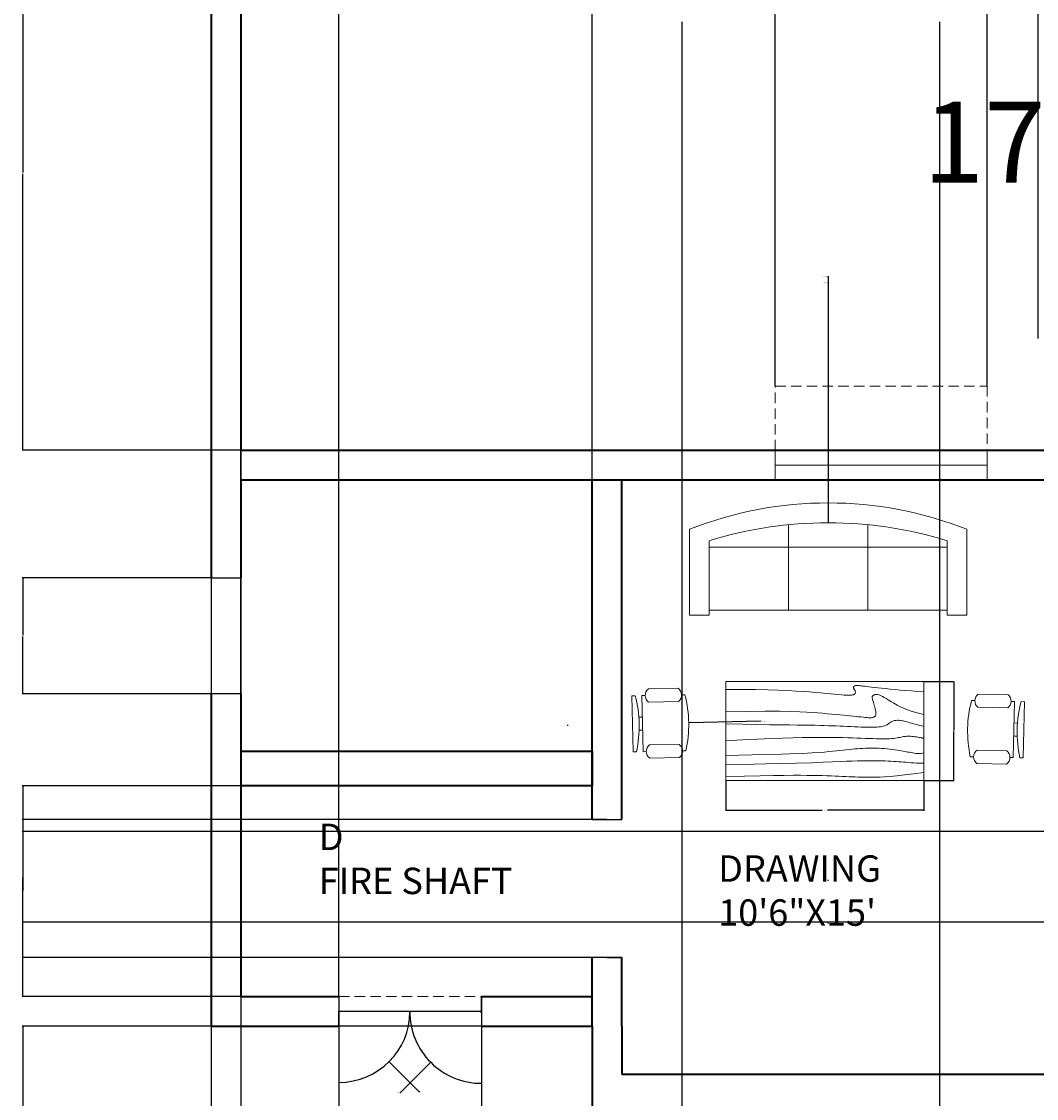
# Model space of a CAD drawing. Units: inches. Extents: x 276 to 912, y -567 to 621.
# Tile 2 of 7: x 276 to 583, y -261 to 65. Entities that reach past the tile are written whole.
import ezdxf

# ---------------------------------------------------------------- set-up
doc = ezdxf.new("R2010")
doc.units = ezdxf.units.IN
doc.linetypes.add('HIDDEN2', pattern=[4.7625, 3.175, -1.5875])
for name, color, linetype, lineweight in [('A-ANNO-DIMS', 2, 'Continuous', 18), ('A-ANNO-TEXT', 7, 'Continuous', 35), ('A-AREA-IDEN', 7, 'Continuous', 18), ('A-DOOR', 3, 'Continuous', 25), ('A-DOOR-HIDN', 3, 'HIDDEN2', 18), ('A-FLOR-OVHD', 8, 'HIDDEN2', 13), ('A-FURN', 8, 'Continuous', 18), ('A-GLAZ', 4, 'Continuous', 18), ('A-WALL', 7, 'Continuous', 35)]:
    doc.layers.add(name, color=color, linetype=linetype, lineweight=lineweight)
doc.dimstyles.get("Standard").update_dxf_attribs({"dimtxt": 0.18, "dimasz": 0.18, "dimexe": 0.18, "dimexo": 0.0625, "dimgap": 0.09, "dimtad": 0, "dimtih": 1, "dimtoh": 1, "dimdec": 4, "dimzin": 0, "dimdsep": 46, "dimtxsty": 'Standard', "dimcen": 0.09, "dimadec": 0, "dimazin": 0, "dimtfac": 1, "dimtdec": 4, "dimtofl": 0, "dimtmove": 0, "dimatfit": 3, "dimfxl": 1, "dimtolj": 1, "dimtzin": 0, "dimarcsym": 0})

# ---------------------------------------------------------------- blocks, each defined once
blk = doc.blocks.new('Table - Rectangular Woodgrain 60 x 30 in.')
for p, q in [((0, 0), (0, -30)), ((60, 0), (0, 0)), ((60, -30), (60, 0)), ((0, -30), (60, -30))]:
    blk.add_line(p, q)
for points in [[(0, -2.4), (4.8155, -2.418), (9.0302, -2.4688), (12.709, -2.5477), (15.9167, -2.65), (18.7181, -2.7711), (21.1781, -2.9063), (23.3616, -3.0508), (25.3333, -3.2), (27.1477, -3.3495), (28.8172, -3.4958), (30.3437, -3.636), (31.7291, -3.7667), (32.9756, -3.8849), (34.0849, -3.9875), (35.059, -4.0714), (35.9, -4.1334), (36.6114, -4.1711), (37.2041, -4.1854), (37.6906, -4.1779), (38.0833, -4.15), (38.3948, -4.1034), (38.6375, -4.0396), (38.8239, -3.9602), (38.9666, -3.8667), (39.0764, -3.7608), (39.1573, -3.6448), (39.2116, -3.521), (39.2416, -3.3917), (39.2498, -3.2593), (39.2385, -3.1261), (39.21, -2.9944), (39.1666, -2.8667), (39.111, -2.7447), (39.0468, -2.6281), (38.978, -2.5163), (38.9083, -2.4083), (38.8418, -2.3035), (38.7823, -2.201), (38.7337, -2.1001), (38.7, -2), (38.6844, -1.9003), (38.6875, -1.8021), (38.7094, -1.707), (38.75, -1.6167), (38.8094, -1.5326), (38.8875, -1.4563), (38.9844, -1.3893), (39.1, -1.3333), (39.2351, -1.2896), (39.3937, -1.2583), (39.5804, -1.2396), (39.8, -1.2333), (40.057, -1.2396), (40.3562, -1.2583), (40.7023, -1.2896), (41.1, -1.3333), (41.5547, -1.3895), (42.0755, -1.4573), (42.6721, -1.5361), (43.3542, -1.625), (44.1316, -1.7233), (45.014, -1.8302), (46.0114, -1.9449), (47.1333, -2.0667), (48.3862, -2.1947), (49.7625, -2.3281), (51.2513, -2.4663), (52.8416, -2.6083), (54.5226, -2.7535), (56.2833, -2.9011), (58.1127, -3.0501), (60, -3.2)], [(0, -9.2), (6.5759, -9.0858), (11.9385, -9.0365), (16.2527, -9.0418), (19.6833, -9.0917), (22.3952, -9.1759), (24.5531, -9.2844), (26.322, -9.4069), (27.8666, -9.5333), (29.3241, -9.6553), (30.7203, -9.7719), (32.0532, -9.8837), (33.3208, -9.9917), (34.5213, -10.0965), (35.6526, -10.199), (36.7128, -10.2999), (37.7, -10.4), (38.6129, -10.4996), (39.4531, -10.5969), (40.223, -10.6895), (40.925, -10.775), (41.5613, -10.8512), (42.1344, -10.9156), (42.6465, -10.966), (43.1, -11), (43.4976, -11.0158), (43.8437, -11.0136), (44.143, -10.9942), (44.4, -10.9583), (44.6195, -10.9069), (44.8062, -10.8406), (44.9648, -10.7603), (45.1, -10.6667), (45.2155, -10.5598), (45.3114, -10.4365), (45.3871, -10.2929), (45.4416, -10.125), (45.4743, -9.929), (45.4844, -9.7011), (45.4709, -9.4371), (45.4333, -9.1333), (45.3716, -8.7883), (45.2896, -8.4104), (45.1919, -8.0107), (45.0833, -7.6), (44.9685, -7.1893), (44.8521, -6.7896), (44.7388, -6.4117), (44.6333, -6.0667), (44.54, -5.7628), (44.4614, -5.4979), (44.4001, -5.2675), (44.3583, -5.0667), (44.3384, -4.8909), (44.3427, -4.7354), (44.3736, -4.5956), (44.4333, -4.4667), (44.5236, -4.3453), (44.6427, -4.2333), (44.7884, -4.1339), (44.9583, -4.05), (45.1501, -3.9849), (45.3614, -3.9417), (45.59, -3.9234), (45.8333, -3.9333), (46.0915, -3.9749), (46.3734, -4.0531), (46.6906, -4.1736), (47.0542, -4.3417), (47.4756, -4.5629), (47.9661, -4.8427), (48.5372, -5.1866), (49.2, -5.6), (49.9676, -6.0844), (50.8594, -6.625), (51.8965, -7.2031), (53.1, -7.8), (54.491, -8.3969), (56.0906, -8.975), (57.9199, -9.5156), (60, -10)], [(0, -12.8), (5.1847, -12.9322), (9.6213, -13.0323), (13.3963, -13.1059), (16.5958, -13.1583), (19.3063, -13.1952), (21.614, -13.2219), (23.6054, -13.2439), (25.3666, -13.2667), (26.9728, -13.2947), (28.4531, -13.3281), (29.8256, -13.3663), (31.1083, -13.4083), (32.3191, -13.4535), (33.476, -13.501), (34.597, -13.5501), (35.7, -13.6), (36.7984, -13.6497), (37.8875, -13.6979), (38.9578, -13.743), (40, -13.7833), (41.0047, -13.8174), (41.9625, -13.8438), (42.864, -13.8607), (43.7, -13.8667), (44.4631, -13.8604), (45.1552, -13.8417), (45.7801, -13.8104), (46.3416, -13.7667), (46.8439, -13.7104), (47.2906, -13.6417), (47.6858, -13.5604), (48.0333, -13.4667), (48.3375, -13.3608), (48.6042, -13.2448), (48.8396, -13.121), (49.05, -12.9917), (49.2417, -12.8593), (49.4208, -12.7261), (49.5937, -12.5944), (49.7667, -12.4667), (49.9452, -12.3451), (50.1323, -12.2313), (50.3303, -12.1268), (50.5416, -12.0333), (50.7686, -11.9524), (51.0135, -11.8854), (51.2788, -11.8341), (51.5666, -11.8), (51.8785, -11.7843), (52.2116, -11.7865), (52.562, -11.8059), (52.926, -11.8417), (53.2998, -11.8931), (53.6795, -11.9594), (54.0614, -12.0397), (54.4416, -12.1333), (54.8223, -12.2401), (55.2293, -12.3625), (55.6942, -12.5037), (56.2489, -12.6667), (56.9251, -12.8547), (57.7545, -13.0708), (58.7689, -13.3182), (60, -13.6)], [(0, -18), (5.124, -17.7273), (9.6609, -17.5057), (13.6705, -17.3303), (17.2125, -17.1958), (20.3467, -17.0973), (23.1328, -17.0297), (25.6307, -16.9878), (27.9, -16.9667), (29.9928, -16.9617), (31.9302, -16.9703), (33.7254, -16.9907), (35.3917, -17.0208), (36.9423, -17.0588), (38.3906, -17.1026), (39.7499, -17.1503), (41.0333, -17.2), (42.2519, -17.2496), (43.4073, -17.2969), (44.4986, -17.3395), (45.525, -17.375), (46.4858, -17.4012), (47.3802, -17.4156), (48.2074, -17.416), (48.9667, -17.4), (49.6583, -17.3662), (50.2872, -17.3167), (50.8595, -17.2547), (51.3812, -17.1833), (51.8584, -17.1057), (52.2971, -17.025), (52.7034, -16.9443), (53.0833, -16.8667), (53.443, -16.7951), (53.789, -16.7313), (54.128, -16.6768), (54.4666, -16.6334), (54.8115, -16.6024), (55.1693, -16.5854), (55.5465, -16.5841), (55.95, -16.6), (56.3828, -16.6337), (56.8346, -16.6823), (57.2915, -16.7418), (57.7396, -16.8084), (58.165, -16.878), (58.5539, -16.9469), (58.8924, -17.0111), (59.1666, -17.0667), (59.3679, -17.1107), (59.5078, -17.1438), (59.6032, -17.1675), (59.6708, -17.1833), (59.7275, -17.193), (59.7901, -17.1979), (59.8753, -17.1998), (60, -17.2)], [(0, -22.4), (8.0098, -22.2501), (14.4094, -22.1011), (19.4168, -21.9535), (23.25, -21.8083), (26.1269, -21.6663), (28.2656, -21.5281), (29.884, -21.3947), (31.2, -21.2667), (32.3967, -21.1448), (33.5172, -21.0292), (34.5697, -20.9198), (35.5625, -20.8167), (36.5037, -20.7198), (37.4015, -20.6292), (38.2642, -20.5448), (39.1, -20.4667), (39.9164, -20.3951), (40.7187, -20.3313), (41.5117, -20.2768), (42.3, -20.2333), (43.0883, -20.2024), (43.8812, -20.1854), (44.6836, -20.1841), (45.5, -20.2), (46.3328, -20.234), (47.1747, -20.2844), (48.0163, -20.3488), (48.8479, -20.425), (49.66, -20.5106), (50.4429, -20.6031), (51.1872, -20.7004), (51.8833, -20.8), (52.5246, -20.8999), (53.1166, -20.9995), (53.6681, -21.0983), (54.1875, -21.1958), (54.6834, -21.2919), (55.1646, -21.3859), (55.6394, -21.4777), (56.1167, -21.5667), (56.6028, -21.6515), (57.0961, -21.7266), (57.5929, -21.7852), (58.0896, -21.8208), (58.5823, -21.8268), (59.0674, -21.7964), (59.5412, -21.723), (60, -21.6)], [(0, -25.2), (8.6355, -25.0504), (15.7026, -24.9031), (21.4049, -24.7606), (25.9458, -24.625), (29.529, -24.4988), (32.3578, -24.3844), (34.6359, -24.284), (36.5667, -24.2), (38.3213, -24.1341), (39.9417, -24.0854), (41.437, -24.0523), (42.8167, -24.0333), (44.0901, -24.0268), (45.2667, -24.0313), (46.3557, -24.0451), (47.3667, -24.0667), (48.309, -24.0947), (49.1928, -24.1287), (50.0284, -24.168), (50.826, -24.2125), (51.5959, -24.2617), (52.3483, -24.3151), (53.0935, -24.3725), (53.8417, -24.4334), (54.6009, -24.497), (55.3699, -24.561), (56.1454, -24.6226), (56.9239, -24.6792), (57.7021, -24.7279), (58.4764, -24.7662), (59.2435, -24.7911), (60, -24.8)], [(0, -28.8), (5.6867, -28.6681), (10.45, -28.5698), (14.407, -28.5012), (17.675, -28.4584), (20.3711, -28.4374), (22.6125, -28.4344), (24.5164, -28.4455), (26.2, -28.4667), (27.762, -28.4947), (29.2276, -28.5281), (30.6033, -28.5663), (31.8958, -28.6084), (33.1118, -28.6535), (34.2578, -28.7011), (35.3405, -28.7501), (36.3666, -28.8), (37.3443, -28.8497), (38.288, -28.8974), (39.2137, -28.9412), (40.1375, -28.9792), (41.0753, -29.0093), (42.0432, -29.0297), (43.0572, -29.0384), (44.1333, -29.0333), (45.2936, -29.0114), (46.5843, -28.9641), (48.0579, -28.8816), (49.7666, -28.7542), (51.7629, -28.5721), (54.0989, -28.3255), (56.8272, -28.0048), (60, -27.6)]]:
    blk.add_lwpolyline(points)
blk = doc.blocks.new('Sofa - Roundback 7 ft.')
for p, q in [((-12.00002, -32.4421), (-12.00003, -6.5971)), ((11.99997, -32.4421), (11.99998, -6.5971)), ((-36.000027, -34), (-36.000027, -11.4696)), ((35.99998, -34), (35.99998, -11.4696)), ((-35.999844, -13.3819), (35.9998, -13.3819)), ((-36.000027, -32.4421), (35.99998, -32.4421))]:
    blk.add_line(p, q)
for points in [[(-36.000027, -34), (-42.000027, -34), (-42.000027, -8)], [(41.99998, -8), (41.99998, -34), (35.99998, -34)]]:
    blk.add_lwpolyline(points)
for centre, radius, start, end in [((0, -114.25), 114.25, 68.43141, 111.5686), ((-0.00001, -127.1968), 121.1968, 72.72033, 107.2797)]:
    blk.add_arc(centre, radius, start, end)
blk = doc.blocks.new('Chair - Desk')
for p, q in [((-8.5, 0), (-8.5, -1)), ((-8.5, 0), (8.5, 0)), ((8.5, 0), (8.5, -1)), ((-8.5, -3), (-8.5, -4)), ((-8.5, -3), (8.5, -3)), ((-2, -3), (-2, -1.9355)), ((2, -1.9576), (2, -3)), ((8.5, -3), (8.5, -4)), ((-10.5, -5), (-10.5, -14)), ((-6.5, -14), (-6.5, -5)), ((6.5, -5), (6.5, -14)), ((10.5, -14), (10.5, -5)), ((-8.5, -15), (-8.5, -16)), ((8.5, -15), (8.5, -16))]:
    blk.add_line(p, q)
for centre, radius, start, end in [((0, 34.625), 36.625, 256.5803, 283.4197), ((-8.5, -6.5), 2.5, 36.8699, 143.1301), ((8.5, -6.5), 2.5, 36.8699, 143.1301), ((-8.5, -12.5), 2.5, 216.8699, 323.1301), ((0, 19.625), 36.625, 256.5803, 283.4197), ((8.5, -12.5), 2.5, 216.8699, 323.1301)]:
    blk.add_arc(centre, radius, start, end)
blk = doc.blocks.new('DOOR-JAMB-9IN')
for p, q in [((4.5, 0), (0, 0)), ((0, 0), (9, 0))]:
    blk.add_line(p, q)
blk = doc.blocks.new('*D22')
at = {"layer": 'A-ANNO-DIMS', "color": 0, "lineweight": -2, "transparency": 16777216}
for p, q in [((488.86, -164.6), (488.86, -173.72)), ((548.86, -164.6), (548.86, -173.72)), ((489.04, -173.54), (518.09, -173.54)), ((548.68, -173.54), (519.62, -173.54))]:
    blk.add_line(p, q, dxfattribs=at)
at = {"layer": 'A-ANNO-DIMS', "color": 0, "transparency": 16777216}
for points in [[(489.04, -173.51), (489.04, -173.57), (488.86, -173.54)], [(548.68, -173.51), (548.68, -173.57), (548.86, -173.54)]]:
    blk.add_solid(points, dxfattribs=at)
at = {"layer": 'Defpoints', "color": 0, "transparency": 16777216}
for p in [(488.86, -164.54), (548.86, -164.54), (548.86, -173.54)]:
    blk.add_point(p, dxfattribs=at)
at = {"layer": 'A-ANNO-DIMS', "color": 0, "transparency": 16777216, "insert": (518.86, -173.54), "char_height": 0.18, "attachment_point": 5}
blk.add_mtext('\\A1;TABLE 60', dxfattribs=at)
blk = doc.blocks.new('*D23')
at = {"layer": 'A-ANNO-DIMS', "color": 0, "lineweight": -2, "transparency": 16777216}
for p, q in [((548.92, -134.54), (558.04, -134.54)), ((557.86, -134.72), (557.86, -149.36)), ((557.86, -164.36), (557.86, -149.72)), ((548.92, -164.54), (558.04, -164.54))]:
    blk.add_line(p, q, dxfattribs=at)
at = {"layer": 'A-ANNO-DIMS', "color": 0, "transparency": 16777216}
for points in [[(557.83, -134.72), (557.89, -134.72), (557.86, -134.54)], [(557.83, -164.36), (557.89, -164.36), (557.86, -164.54)]]:
    blk.add_solid(points, dxfattribs=at)
at = {"layer": 'Defpoints', "color": 0, "transparency": 16777216}
for p in [(548.86, -134.54), (557.86, -134.54), (548.86, -164.54)]:
    blk.add_point(p, dxfattribs=at)
at = {"layer": 'A-ANNO-DIMS', "color": 0, "transparency": 16777216, "insert": (557.86, -149.54), "char_height": 0.18, "attachment_point": 5}
blk.add_mtext('\\A1;30', dxfattribs=at)
blk = doc.blocks.new('*D24')
at = {"layer": 'A-ANNO-DIMS', "color": 0, "lineweight": -2, "transparency": 16777216}
for p, q in [((333.082179, 103.255751), (333.082179, -553.223061)), ((854.209085, -327.604004), (854.209085, -553.223061)), ((333.262179, -553.043061), (593.255632, -553.043061)), ((854.029085, -553.043061), (594.035632, -553.043061))]:
    blk.add_line(p, q, dxfattribs=at)
at = {"layer": 'A-ANNO-DIMS', "color": 0, "transparency": 16777216}
for points in [[(333.262179, -553.013061), (333.262179, -553.073061), (333.082179, -553.043061)], [(854.029085, -553.013061), (854.029085, -553.073061), (854.209085, -553.043061)]]:
    blk.add_solid(points, dxfattribs=at)
at = {"layer": 'Defpoints', "color": 0, "transparency": 16777216}
for p in [(333.082179, 103.318251), (854.209085, -327.541504), (854.209085, -553.043061)]:
    blk.add_point(p, dxfattribs=at)
at = {"layer": 'A-ANNO-DIMS', "color": 0, "transparency": 16777216, "insert": (593.645632, -553.043061), "char_height": 0.18, "attachment_point": 5}
blk.add_mtext('\\A1;521.1', dxfattribs=at)
blk = doc.blocks.new('*D25')
at = {"layer": 'A-ANNO-DIMS', "color": 0, "lineweight": -2, "transparency": 16777216}
for p, q in [((478.5, 564.29), (911.39, 564.29)), ((911.21, 564.11), (911.21, 34.31)), ((911.21, -495.86), (911.21, 33.95)), ((582.98, -496.04), (911.39, -496.04))]:
    blk.add_line(p, q, dxfattribs=at)
at = {"layer": 'A-ANNO-DIMS', "color": 0, "transparency": 16777216}
for points in [[(911.18, 564.11), (911.24, 564.11), (911.21, 564.29)], [(911.18, -495.86), (911.24, -495.86), (911.21, -496.04)]]:
    blk.add_solid(points, dxfattribs=at)
at = {"layer": 'Defpoints', "color": 0, "transparency": 16777216}
for p in [(478.44, 564.29), (582.92, -496.04), (911.21, -496.04)]:
    blk.add_point(p, dxfattribs=at)
at = {"layer": 'A-ANNO-DIMS', "color": 0, "transparency": 16777216, "insert": (911.21, 34.13), "char_height": 0.18, "attachment_point": 5}
blk.add_mtext('\\A1;1060.3', dxfattribs=at)
blk = doc.blocks.new('*D26')
at = {"layer": 'A-ANNO-DIMS', "color": 0, "lineweight": -2, "transparency": 16777216}
for p, q in [((342.02, 103.32), (275.9, 103.32)), ((276.08, 103.14), (276.08, 19.57)), ((276.08, -64.36), (276.08, 19.21)), ((342.02, -64.54), (275.9, -64.54))]:
    blk.add_line(p, q, dxfattribs=at)
at = {"layer": 'A-ANNO-DIMS', "color": 0, "transparency": 16777216}
for points in [[(276.05, 103.14), (276.11, 103.14), (276.08, 103.32)], [(276.05, -64.36), (276.11, -64.36), (276.08, -64.54)]]:
    blk.add_solid(points, dxfattribs=at)
at = {"layer": 'Defpoints', "color": 0, "transparency": 16777216}
for p in [(342.08, 103.32), (276.08, -64.54), (342.08, -64.54)]:
    blk.add_point(p, dxfattribs=at)
at = {"layer": 'A-ANNO-DIMS', "color": 0, "transparency": 16777216, "insert": (276.08, 19.39), "char_height": 0.18, "attachment_point": 5}
blk.add_mtext('\\A1;167.86', dxfattribs=at)
blk = doc.blocks.new('*D31')
at = {"layer": 'A-ANNO-DIMS', "color": 0, "lineweight": -2, "transparency": 16777216}
for p, q in [((333.082179, 103.255751), (333.082179, -553.223061)), ((475.582179, 65.246155), (475.582179, -553.223061)), ((333.262179, -553.043061), (403.912179, -553.043061)), ((475.402179, -553.043061), (404.752179, -553.043061))]:
    blk.add_line(p, q, dxfattribs=at)
at = {"layer": 'A-ANNO-DIMS', "color": 0, "transparency": 16777216}
for points in [[(333.262179, -553.013061), (333.262179, -553.073061), (333.082179, -553.043061)], [(475.402179, -553.013061), (475.402179, -553.073061), (475.582179, -553.043061)]]:
    blk.add_solid(points, dxfattribs=at)
at = {"layer": 'Defpoints', "color": 0, "transparency": 16777216}
for p in [(333.082179, 103.318251), (475.582179, 65.308655), (475.582179, -553.043061)]:
    blk.add_point(p, dxfattribs=at)
at = {"layer": 'A-ANNO-DIMS', "color": 0, "transparency": 16777216, "insert": (404.332179, -553.043061), "char_height": 0.18, "attachment_point": 5}
blk.add_mtext('\\A1;142.5', dxfattribs=at)
blk = doc.blocks.new('*D32')
at = {"layer": 'A-ANNO-DIMS', "color": 0, "lineweight": -2, "transparency": 16777216}
for p, q in [((475.582179, 65.246155), (475.582179, -553.223061)), ((553.582179, 65.246155), (553.582179, -553.223061)), ((475.762179, -553.043061), (514.342179, -553.043061)), ((553.402179, -553.043061), (514.822179, -553.043061))]:
    blk.add_line(p, q, dxfattribs=at)
at = {"layer": 'A-ANNO-DIMS', "color": 0, "transparency": 16777216}
for points in [[(475.762179, -553.013061), (475.762179, -553.073061), (475.582179, -553.043061)], [(553.402179, -553.013061), (553.402179, -553.073061), (553.582179, -553.043061)]]:
    blk.add_solid(points, dxfattribs=at)
at = {"layer": 'Defpoints', "color": 0, "transparency": 16777216}
for p in [(475.582179, 65.308655), (553.582179, 65.308655), (553.582179, -553.043061)]:
    blk.add_point(p, dxfattribs=at)
at = {"layer": 'A-ANNO-DIMS', "color": 0, "transparency": 16777216, "insert": (514.582179, -553.043061), "char_height": 0.18, "attachment_point": 5}
blk.add_mtext('\\A1;78', dxfattribs=at)
blk = doc.blocks.new('*D33')
at = {"layer": 'A-ANNO-DIMS', "color": 0, "lineweight": -2, "transparency": 16777216}
for p, q in [((553.582179, 65.246155), (553.582179, -553.223061)), ((668.582179, 65.246155), (668.582179, -553.223061)), ((553.762179, -553.043061), (610.812179, -553.043061)), ((668.402179, -553.043061), (611.352179, -553.043061))]:
    blk.add_line(p, q, dxfattribs=at)
at = {"layer": 'A-ANNO-DIMS', "color": 0, "transparency": 16777216}
for points in [[(553.762179, -553.013061), (553.762179, -553.073061), (553.582179, -553.043061)], [(668.402179, -553.013061), (668.402179, -553.073061), (668.582179, -553.043061)]]:
    blk.add_solid(points, dxfattribs=at)
at = {"layer": 'Defpoints', "color": 0, "transparency": 16777216}
for p in [(553.582179, 65.308655), (668.582179, 65.308655), (668.582179, -553.043061)]:
    blk.add_point(p, dxfattribs=at)
at = {"layer": 'A-ANNO-DIMS', "color": 0, "transparency": 16777216, "insert": (611.082179, -553.043061), "char_height": 0.18, "attachment_point": 5}
blk.add_mtext('\\A1;115', dxfattribs=at)
blk = doc.blocks.new('*D41')
at = {"layer": 'A-ANNO-DIMS', "color": 0, "lineweight": -2, "transparency": 16777216}
for p, q in [((333.082179, 363.769143), (333.082179, -553.223061)), ((342.082179, 363.769143), (342.082179, -553.223061)), ((333.262179, -553.043061), (337.432179, -553.043061)), ((341.902179, -553.043061), (337.732179, -553.043061))]:
    blk.add_line(p, q, dxfattribs=at)
at = {"layer": 'A-ANNO-DIMS', "color": 0, "transparency": 16777216}
for points in [[(333.262179, -553.013061), (333.262179, -553.073061), (333.082179, -553.043061)], [(341.902179, -553.013061), (341.902179, -553.073061), (342.082179, -553.043061)]]:
    blk.add_solid(points, dxfattribs=at)
at = {"layer": 'Defpoints', "color": 0, "transparency": 16777216}
for p in [(333.082179, 363.831643), (342.082179, 363.831643), (342.082179, -553.043061)]:
    blk.add_point(p, dxfattribs=at)
at = {"layer": 'A-ANNO-DIMS', "color": 0, "transparency": 16777216, "insert": (337.582179, -553.043061), "char_height": 0.18, "attachment_point": 5}
blk.add_mtext('\\A1;9', dxfattribs=at)
blk = doc.blocks.new('*D55')
at = {"layer": 'A-ANNO-DIMS', "color": 0, "lineweight": -2, "transparency": 16777216}
for p, q in [((333.082179, -239.052429), (333.082179, -553.223061)), ((448.418489, -454.604004), (448.418489, -553.223061)), ((333.262179, -553.043061), (390.270334, -553.043061)), ((448.238489, -553.043061), (391.230334, -553.043061))]:
    blk.add_line(p, q, dxfattribs=at)
at = {"layer": 'A-ANNO-DIMS', "color": 0, "transparency": 16777216}
for points in [[(333.262179, -553.013061), (333.262179, -553.073061), (333.082179, -553.043061)], [(448.238489, -553.013061), (448.238489, -553.073061), (448.418489, -553.043061)]]:
    blk.add_solid(points, dxfattribs=at)
at = {"layer": 'Defpoints', "color": 0, "transparency": 16777216}
for p in [(333.082179, -238.989929), (448.418489, -454.541504), (448.418489, -553.043061)]:
    blk.add_point(p, dxfattribs=at)
at = {"layer": 'A-ANNO-DIMS', "color": 0, "transparency": 16777216, "insert": (390.750334, -553.043061), "char_height": 0.18, "attachment_point": 5}
blk.add_mtext('\\A1;115.34', dxfattribs=at)
blk = doc.blocks.new('*D59')
at = {"layer": 'A-ANNO-DIMS', "color": 0, "lineweight": -2, "transparency": 16777216}
for p, q in [((333.082179, -81.315568), (333.082179, 621.473746)), ((333.262179, 621.293746), (457.725334, 621.293746)), ((583.238489, 621.293746), (458.775334, 621.293746)), ((583.418489, -30.671128), (583.418489, 621.473746))]:
    blk.add_line(p, q, dxfattribs=at)
at = {"layer": 'A-ANNO-DIMS', "color": 0, "transparency": 16777216}
for points in [[(333.262179, 621.323746), (333.262179, 621.263746), (333.082179, 621.293746)], [(583.238489, 621.323746), (583.238489, 621.263746), (583.418489, 621.293746)]]:
    blk.add_solid(points, dxfattribs=at)
at = {"layer": 'Defpoints', "color": 0, "transparency": 16777216}
for p in [(583.418489, 621.293746), (583.418489, -30.733628), (333.082179, -81.378068)]:
    blk.add_point(p, dxfattribs=at)
at = {"layer": 'A-ANNO-DIMS', "color": 0, "transparency": 16777216, "insert": (458.250334, 621.293746), "char_height": 0.18, "attachment_point": 5}
blk.add_mtext('\\A1;250.34', dxfattribs=at)
blk = doc.blocks.new('*D64')
at = {"layer": 'A-ANNO-DIMS', "color": 0, "lineweight": -2, "transparency": 16777216}
for p, q in [((371.772434, -239.052429), (371.772434, -553.223061)), ((414.936626, -239.052429), (414.936626, -553.223061)), ((371.952434, -553.043061), (392.93453, -553.043061)), ((414.756626, -553.043061), (393.77453, -553.043061))]:
    blk.add_line(p, q, dxfattribs=at)
at = {"layer": 'A-ANNO-DIMS', "color": 0, "transparency": 16777216}
for points in [[(371.952434, -553.013061), (371.952434, -553.073061), (371.772434, -553.043061)], [(414.756626, -553.013061), (414.756626, -553.073061), (414.936626, -553.043061)]]:
    blk.add_solid(points, dxfattribs=at)
at = {"layer": 'Defpoints', "color": 0, "transparency": 16777216}
for p in [(371.772434, -238.989929), (414.936626, -238.989929), (414.936626, -553.043061)]:
    blk.add_point(p, dxfattribs=at)
at = {"layer": 'A-ANNO-DIMS', "color": 0, "transparency": 16777216, "insert": (393.35453, -553.043061), "char_height": 0.18, "attachment_point": 5}
blk.add_mtext('\\A1;43.16', dxfattribs=at)
blk = doc.blocks.new('*D65')
at = {"layer": 'A-ANNO-DIMS', "color": 0, "lineweight": -2, "transparency": 16777216}
for p, q in [((342.08, -229.93), (342.08, 621.47)), ((342.26, 621.29), (356.48, 621.29)), ((371.59, 621.29), (357.38, 621.29)), ((371.77, -229.93), (371.77, 621.47))]:
    blk.add_line(p, q, dxfattribs=at)
at = {"layer": 'A-ANNO-DIMS', "color": 0, "transparency": 16777216}
for points in [[(342.26, 621.32), (342.26, 621.26), (342.08, 621.29)], [(371.59, 621.32), (371.59, 621.26), (371.77, 621.29)]]:
    blk.add_solid(points, dxfattribs=at)
at = {"layer": 'Defpoints', "color": 0, "transparency": 16777216}
for p in [(371.77, 621.29), (342.08, -229.99), (371.77, -229.99)]:
    blk.add_point(p, dxfattribs=at)
at = {"layer": 'A-ANNO-DIMS', "color": 0, "transparency": 16777216, "insert": (356.93, 621.29), "char_height": 0.18, "attachment_point": 5}
blk.add_mtext('\\A1;29.69', dxfattribs=at)
blk = doc.blocks.new('*D66')
at = {"layer": 'A-ANNO-DIMS', "color": 0, "lineweight": -2, "transparency": 16777216}
for p, q in [((342.02, -166.15), (275.9, -166.15)), ((276.08, -166.33), (276.08, -197.89)), ((276.08, -229.81), (276.08, -198.25)), ((342.02, -229.99), (275.9, -229.99))]:
    blk.add_line(p, q, dxfattribs=at)
at = {"layer": 'A-ANNO-DIMS', "color": 0, "transparency": 16777216}
for points in [[(276.05, -166.33), (276.11, -166.33), (276.08, -166.15)], [(276.05, -229.81), (276.11, -229.81), (276.08, -229.99)]]:
    blk.add_solid(points, dxfattribs=at)
at = {"layer": 'Defpoints', "color": 0, "transparency": 16777216}
for p in [(342.08, -166.15), (276.08, -229.99), (342.08, -229.99)]:
    blk.add_point(p, dxfattribs=at)
at = {"layer": 'A-ANNO-DIMS', "color": 0, "transparency": 16777216, "insert": (276.08, -198.07), "char_height": 0.18, "attachment_point": 5}
blk.add_mtext('\\A1;63.84', dxfattribs=at)
blk = doc.blocks.new('*D67')
at = {"layer": 'A-ANNO-DIMS', "color": 0, "lineweight": -2, "transparency": 16777216}
for p, q in [((448.36, -176.33), (275.9, -176.33)), ((276.08, -176.51), (276.08, -197.09)), ((276.08, -218.02), (276.08, -197.45)), ((448.36, -218.2), (275.9, -218.2))]:
    blk.add_line(p, q, dxfattribs=at)
at = {"layer": 'A-ANNO-DIMS', "color": 0, "transparency": 16777216}
for points in [[(276.05, -176.51), (276.11, -176.51), (276.08, -176.33)], [(276.05, -218.02), (276.11, -218.02), (276.08, -218.2)]]:
    blk.add_solid(points, dxfattribs=at)
at = {"layer": 'Defpoints', "color": 0, "transparency": 16777216}
for p in [(448.42, -176.33), (276.08, -218.2), (448.42, -218.2)]:
    blk.add_point(p, dxfattribs=at)
at = {"layer": 'A-ANNO-DIMS', "color": 0, "transparency": 16777216, "insert": (276.08, -197.27), "char_height": 0.18, "attachment_point": 5}
blk.add_mtext('\\A1;41.866', dxfattribs=at)
blk = doc.blocks.new('*D69')
at = {"layer": 'A-ANNO-DIMS', "color": 0, "lineweight": -2, "transparency": 16777216}
for p, q in [((592.355989, -180.041504), (275.902179, -180.041504)), ((276.082179, -180.221504), (276.082179, -193.59361)), ((276.082179, -207.325716), (276.082179, -193.95361)), ((592.355989, -207.505716), (275.902179, -207.505716))]:
    blk.add_line(p, q, dxfattribs=at)
at = {"layer": 'A-ANNO-DIMS', "color": 0, "transparency": 16777216}
for points in [[(276.052179, -180.221504), (276.112179, -180.221504), (276.082179, -180.041504)], [(276.052179, -207.325716), (276.112179, -207.325716), (276.082179, -207.505716)]]:
    blk.add_solid(points, dxfattribs=at)
at = {"layer": 'Defpoints', "color": 0, "transparency": 16777216}
for p in [(276.082179, -180.041504), (592.418489, -180.041504), (592.418489, -207.505716)]:
    blk.add_point(p, dxfattribs=at)
at = {"layer": 'A-ANNO-DIMS', "color": 0, "transparency": 16777216, "insert": (276.082179, -193.77361), "char_height": 0.18, "attachment_point": 5}
blk.add_mtext('\\A1;27.464', dxfattribs=at)
blk = doc.blocks.new('*D70')
at = {"layer": 'A-ANNO-DIMS', "color": 0, "lineweight": -2, "transparency": 16777216}
for p, q in [((448.42, -73.48), (448.42, 621.47)), ((448.6, 621.29), (475.69, 621.29)), ((503.69, 621.29), (476.59, 621.29)), ((503.87, -45.06), (503.87, 621.47))]:
    blk.add_line(p, q, dxfattribs=at)
at = {"layer": 'A-ANNO-DIMS', "color": 0, "transparency": 16777216}
for points in [[(448.6, 621.32), (448.6, 621.26), (448.42, 621.29)], [(503.69, 621.32), (503.69, 621.26), (503.87, 621.29)]]:
    blk.add_solid(points, dxfattribs=at)
at = {"layer": 'Defpoints', "color": 0, "transparency": 16777216}
for p in [(503.87, 621.29), (503.87, -45.12), (448.42, -73.54)]:
    blk.add_point(p, dxfattribs=at)
at = {"layer": 'A-ANNO-DIMS', "color": 0, "transparency": 16777216, "insert": (476.14, 621.29), "char_height": 0.18, "attachment_point": 5}
blk.add_mtext('\\A1;55.45', dxfattribs=at)
blk = doc.blocks.new('*D71')
at = {"layer": 'A-ANNO-DIMS', "color": 0, "lineweight": -2, "transparency": 16777216}
for p, q in [((503.866476, -45.059003), (503.866476, 621.473746)), ((504.046476, 621.293746), (535.522963, 621.293746)), ((567.83945, 621.293746), (536.362963, 621.293746)), ((568.01945, -45.059003), (568.01945, 621.473746))]:
    blk.add_line(p, q, dxfattribs=at)
at = {"layer": 'A-ANNO-DIMS', "color": 0, "transparency": 16777216}
for points in [[(504.046476, 621.323746), (504.046476, 621.263746), (503.866476, 621.293746)], [(567.83945, 621.323746), (567.83945, 621.263746), (568.01945, 621.293746)]]:
    blk.add_solid(points, dxfattribs=at)
at = {"layer": 'Defpoints', "color": 0, "transparency": 16777216}
for p in [(568.01945, 621.293746), (503.866476, -45.121503), (568.01945, -45.121503)]:
    blk.add_point(p, dxfattribs=at)
at = {"layer": 'A-ANNO-DIMS', "color": 0, "transparency": 16777216, "insert": (535.942963, 621.293746), "char_height": 0.18, "attachment_point": 5}
blk.add_mtext('\\A1;64.15', dxfattribs=at)
blk = doc.blocks.new('*D74')
at = {"layer": 'A-ANNO-DIMS', "color": 0, "lineweight": -2, "transparency": 16777216}
for p, q in [((333.019679, -103.210426), (275.902179, -103.210426)), ((276.082179, -103.390426), (276.082179, -120.559631)), ((276.082179, -138.088836), (276.082179, -120.919631)), ((333.019679, -138.268836), (275.902179, -138.268836))]:
    blk.add_line(p, q, dxfattribs=at)
at = {"layer": 'A-ANNO-DIMS', "color": 0, "transparency": 16777216}
for points in [[(276.052179, -103.390426), (276.112179, -103.390426), (276.082179, -103.210426)], [(276.052179, -138.088836), (276.112179, -138.088836), (276.082179, -138.268836)]]:
    blk.add_solid(points, dxfattribs=at)
at = {"layer": 'Defpoints', "color": 0, "transparency": 16777216}
for p in [(333.082179, -103.210426), (276.082179, -138.268836), (333.082179, -138.268836)]:
    blk.add_point(p, dxfattribs=at)
at = {"layer": 'A-ANNO-DIMS', "color": 0, "transparency": 16777216, "insert": (276.082179, -120.739631), "char_height": 0.18, "attachment_point": 5}
blk.add_mtext('\\A1;35.06', dxfattribs=at)
blk = doc.blocks.new('*D75')
at = {"layer": 'A-ANNO-DIMS', "color": 0, "lineweight": -2, "transparency": 16777216}
for p, q in [((448.36, -238.99), (275.9, -238.99)), ((276.08, -239.17), (276.08, -346.59)), ((276.08, -454.36), (276.08, -346.95)), ((448.36, -454.54), (275.9, -454.54))]:
    blk.add_line(p, q, dxfattribs=at)
at = {"layer": 'A-ANNO-DIMS', "color": 0, "transparency": 16777216}
for points in [[(276.05, -239.17), (276.11, -239.17), (276.08, -238.99)], [(276.05, -454.36), (276.11, -454.36), (276.08, -454.54)]]:
    blk.add_solid(points, dxfattribs=at)
at = {"layer": 'Defpoints', "color": 0, "transparency": 16777216}
for p in [(276.08, -238.99), (448.42, -238.99), (448.42, -454.54)]:
    blk.add_point(p, dxfattribs=at)
at = {"layer": 'A-ANNO-DIMS', "color": 0, "transparency": 16777216, "insert": (276.08, -346.77), "char_height": 0.18, "attachment_point": 5}
blk.add_mtext('\\A1;215.55', dxfattribs=at)
blk = doc.blocks.new('*D79')
at = {"layer": 'A-ANNO-DIMS', "color": 0, "lineweight": -2, "transparency": 16777216}
for p, q in [((371.68, -234.49), (371.86, -234.49)), ((371.77, -234.58), (371.77, -234.4)), ((396.1, -258.81), (387.1, -249.82)), ((396.28, -258.81), (396.1, -258.81))]:
    blk.add_line(p, q, dxfattribs=at)
at = {"layer": 'A-ANNO-DIMS', "color": 0, "transparency": 16777216}
blk.add_solid([(387.12, -249.8), (387.08, -249.84), (386.98, -249.69)], dxfattribs=at)
at = {"layer": 'Defpoints', "color": 0, "transparency": 16777216}
for p in [(371.77, -234.49), (386.98, -249.69)]:
    blk.add_point(p, dxfattribs=at)
at = {"layer": 'A-ANNO-DIMS', "color": 0, "transparency": 16777216, "insert": (396.7, -258.81), "char_height": 0.18, "attachment_point": 5}
blk.add_mtext('\\A1;R21.5', dxfattribs=at)
blk = doc.blocks.new('*D80')
at = {"layer": 'A-ANNO-DIMS', "color": 0, "lineweight": -2, "transparency": 16777216}
for p, q in [((414.77, -234.68), (414.95, -234.68)), ((414.86, -234.77), (414.86, -234.59)), ((390.37, -259.04), (399.43, -250.03)), ((390.19, -259.04), (390.37, -259.04))]:
    blk.add_line(p, q, dxfattribs=at)
at = {"layer": 'A-ANNO-DIMS', "color": 0, "transparency": 16777216}
blk.add_solid([(399.41, -250.01), (399.45, -250.05), (399.55, -249.9)], dxfattribs=at)
at = {"layer": 'Defpoints', "color": 0, "transparency": 16777216}
for p in [(414.86, -234.68), (399.55, -249.9)]:
    blk.add_point(p, dxfattribs=at)
at = {"layer": 'A-ANNO-DIMS', "color": 0, "transparency": 16777216, "insert": (389.59, -259.04), "char_height": 0.18, "attachment_point": 5}
blk.add_mtext('\\A1;R21.587', dxfattribs=at)
blk = doc.blocks.new('*D81')
at = {"layer": 'A-ANNO-DIMS', "color": 0, "lineweight": -2, "transparency": 16777216}
for p, q in [((519.69, -13.76), (519.87, -13.76)), ((519.87, -13.76), (519.87, -86.3)), ((519.79, -207.68), (519.97, -207.68)), ((519.88, -207.77), (519.88, -207.59))]:
    blk.add_line(p, q, dxfattribs=at)
at = {"layer": 'A-ANNO-DIMS', "color": 0, "transparency": 16777216}
blk.add_solid([(519.9, -86.3), (519.84, -86.3), (519.87, -86.48)], dxfattribs=at)
at = {"layer": 'Defpoints', "color": 0, "transparency": 16777216}
for p in [(519.87, -86.48), (519.88, -207.68)]:
    blk.add_point(p, dxfattribs=at)
at = {"layer": 'A-ANNO-DIMS', "color": 0, "transparency": 16777216, "insert": (518.94, -13.76), "char_height": 0.18, "attachment_point": 5}
blk.add_mtext('\\A1;2X R121.2', dxfattribs=at)
blk = doc.blocks.new('*D82')
at = {"layer": 'A-ANNO-DIMS', "color": 0, "lineweight": -2, "transparency": 16777216}
for p, q in [((519.69, -11.93), (519.87, -11.93)), ((519.87, -11.93), (519.87, -80.3)), ((519.79, -194.73), (519.97, -194.73)), ((519.88, -194.82), (519.88, -194.64))]:
    blk.add_line(p, q, dxfattribs=at)
at = {"layer": 'A-ANNO-DIMS', "color": 0, "transparency": 16777216}
blk.add_solid([(519.9, -80.3), (519.84, -80.3), (519.87, -80.48)], dxfattribs=at)
at = {"layer": 'Defpoints', "color": 0, "transparency": 16777216}
for p in [(519.87, -80.48), (519.88, -194.73)]:
    blk.add_point(p, dxfattribs=at)
at = {"layer": 'A-ANNO-DIMS', "color": 0, "transparency": 16777216, "insert": (518.85, -11.93), "char_height": 0.18, "attachment_point": 5}
blk.add_mtext('\\A1;2X R114.25', dxfattribs=at)
blk = doc.blocks.new('*D83')
at = {"layer": 'A-ANNO-DIMS', "color": 0, "lineweight": -2, "transparency": 16777216}
for p, q in [((499.62, -146.62), (477.83, -147.05)), ((440.94, -147.78), (441.12, -147.78)), ((441.03, -147.87), (441.03, -147.69))]:
    blk.add_line(p, q, dxfattribs=at)
at = {"layer": 'A-ANNO-DIMS', "color": 0, "transparency": 16777216}
blk.add_solid([(477.83, -147.02), (477.83, -147.08), (477.65, -147.06)], dxfattribs=at)
at = {"layer": 'Defpoints', "color": 0, "transparency": 16777216}
for p in [(441.03, -147.78), (477.65, -147.06)]:
    blk.add_point(p, dxfattribs=at)
at = {"layer": 'A-ANNO-DIMS', "color": 0, "transparency": 16777216, "insert": (500.52, -146.62), "char_height": 0.18, "attachment_point": 5}
blk.add_mtext('\\A1;2X R36.625', dxfattribs=at)

msp = doc.modelspace()

# ---------------------------------------------------------------- linework, layer by layer
at = {"layer": 'A-DOOR'}
for p, q in [((333.0822, -103.2104), (342.0822, -103.2104)), ((342.0822, -138.2688), (333.0822, -138.2688)), ((371.7724, -229.9899), (371.7724, -238.9899)), ((414.9366, -234.4899), (414.9366, -229.9899)), ((414.9366, -229.9899), (414.9366, -238.9899)), ((371.7724, -238.9899), (371.7724, -234.4899)), ((414.9366, -234.4899), (371.7724, -234.4899)), ((371.7724, -234.4899), (371.7724, -255.9893)), ((414.9366, -234.4899), (414.9366, -256.2665))]:
    msp.add_line(p, q, dxfattribs=at)
for centre, radius, start, end in [((371.7724, -234.4899), 21.4993, 270, 0), ((414.8581, -234.6795), 21.5872, 179.496822, 270.208421)]:
    msp.add_arc(centre, radius, start, end, dxfattribs=at)
at = {"layer": 'A-DOOR-HIDN'}
for p, q in [((448.4185, -218.1988), (457.4185, -218.1988)), ((371.7724, -229.9899), (414.9366, -229.9899))]:
    msp.add_line(p, q, dxfattribs=at)
at = {"layer": 'A-FLOR-OVHD'}
for p, q in [((503.8665, -64.5415), (503.8665, -45.1215)), ((503.8665, -45.1215), (568.0194, -45.1215)), ((568.0194, -45.1215), (568.0194, -64.5415))]:
    msp.add_line(p, q, dxfattribs=at)
at = {"layer": 'A-GLAZ'}
for p, q in [((503.8665, -69.0415), (503.8665, -64.5415)), ((503.8665, -64.5415), (503.8665, -73.5415)), ((568.0194, -64.5415), (568.0194, -73.5415)), ((568.0194, -69.0415), (503.8665, -69.0415))]:
    msp.add_line(p, q, dxfattribs=at)
at = {"layer": 'A-WALL'}
for p, q in [((333.0822, 103.3183), (333.0822, -81.3781)), ((342.0822, 103.3183), (342.0822, -64.5415)), ((342.0822, -64.5415), (821.9185, -64.5415)), ((342.0822, -73.5415), (812.9185, -73.5415)), ((342.0822, -73.5415), (342.0822, -81.3781)), ((448.4185, -176.3331), (448.4185, -73.5415)), ((457.4185, -176.3331), (457.4185, -73.5415)), ((333.0822, -81.3781), (333.0822, -103.2104)), ((342.0822, -81.3781), (342.0822, -103.2104)), ((333.0822, -138.2688), (333.0822, -238.9899)), ((342.0822, -138.2688), (342.0822, -229.9899)), ((342.0822, -155.684), (448.4185, -155.684)), ((448.4185, -155.684), (448.4185, -166.1493)), ((448.4185, -166.1493), (342.0822, -166.1493)), ((448.4185, -238.9899), (448.4185, -218.1988)), ((457.4185, -238.9899), (457.4185, -218.1988)), ((342.0822, -229.9899), (371.7724, -229.9899)), ((414.9366, -229.9899), (448.4185, -229.9899)), ((333.0822, -238.9899), (371.7724, -238.9899)), ((414.9366, -238.9899), (448.4185, -238.9899)), ((448.4185, -238.9899), (448.4185, -454.5415)), ((457.4185, -238.9899), (457.4185, -253.5415)), ((457.4185, -253.5415), (592.4185, -253.5415))]:
    msp.add_line(p, q, dxfattribs=at)

# ---------------------------------------------------------------- block references
at = {"layer": 'A-DOOR'}
msp.add_blockref('DOOR-JAMB-9IN', (448.4183, -176.3328), dxfattribs=at)
at = {"layer": 'A-DOOR', "rotation": 180}
msp.add_blockref('DOOR-JAMB-9IN', (457.4187, -218.1991), dxfattribs=at)
at = {"layer": 'A-FURN'}
for name, p in [('Sofa - Roundback 7 ft.', (519.8751, -80.4825)), ('Table - Rectangular Woodgrain 60 x 30 in.', (488.8572, -134.5418))]:
    msp.add_blockref(name, p, dxfattribs=at)
at = {"layer": 'A-FURN', "rotation": 91.13258359851098}
msp.add_blockref('Chair - Desk', (460.6556, -147.3921), dxfattribs=at)
at = {"layer": 'A-FURN', "xscale": -1, "rotation": 268.7664642392211}
msp.add_blockref('Chair - Desk', (579.0823, -149.188), dxfattribs=at)

# ---------------------------------------------------------------- texts
at = {"layer": 'A-ANNO-TEXT', "insert": (548.5415, 41.0446), "char_height": 24.49138, "attachment_point": 1}
msp.add_mtext_dynamic_manual_height_columns('{\\fTimes New Roman|b0|i0|c0|p18;1741SFT}', width=190.647076, gutter_width=38.2678, heights=[0], dxfattribs=at)
at = {"layer": 'A-AREA-IDEN', "char_height": 8, "attachment_point": 1}
for s, insert in [('{\\fTimes New Roman|b0|i0|c0|p18;D\\PFIRE SHAFT}', (365.6579, -177.6222)), ('{\\fTimes New Roman|b0|i0|c0|p18;DRAWING\\P10\'6"X15\'}', (486.5832, -187.2193))]:
    msp.add_mtext_dynamic_manual_height_columns(s, width=62.274017, gutter_width=12.5, heights=[0], dxfattribs=dict(at, insert=insert))

# ---------------------------------------------------------------- dimensions: what is measured, and where the dimension line sits
at = {"layer": 'A-ANNO-DIMS'}
for base, p1, p2, override, picture, middle in [((583.4185, 621.2937), (333.0822, -81.3781), (583.4185, -30.7336), {"dimdec": 2, "dimlfac": 1, "dimrnd": 0, "dimzin": 0, "dimdsep": 46, "dimlunit": 2}, '*D59', (458.2503, 621.2937)), ((371.7724, 621.2937), (342.0822, -229.9899), (371.7724, -229.9899), {"dimdec": 2, "dimlfac": 1, "dimrnd": 0, "dimzin": 0, "dimdsep": 46, "dimlunit": 2}, '*D65', (356.9273, 621.2937)), ((503.8665, 621.2937), (448.4185, -73.5415), (503.8665, -45.1215), {"dimdec": 2, "dimlfac": 1, "dimrnd": 0, "dimzin": 0, "dimdsep": 46, "dimlunit": 2}, '*D70', (476.1425, 621.2937)), ((568.0194, 621.2937), (503.8665, -45.1215), (568.0194, -45.1215), {"dimdec": 2, "dimlfac": 1, "dimrnd": 0, "dimzin": 0, "dimdsep": 46, "dimlunit": 2}, '*D71', (535.943, 621.2937)), ((342.0822, -553.0431), (333.0822, 363.8316), (342.0822, 363.8316), {"dimdec": 0, "dimlfac": 1, "dimrnd": 0, "dimzin": 0, "dimdsep": 46, "dimlunit": 2}, '*D41', (337.5822, -553.0431)), ((854.2091, -553.0431), (333.0822, 103.3183), (854.2091, -327.5415), {"dimdec": 1, "dimlfac": 1, "dimrnd": 0, "dimzin": 0, "dimdsep": 46, "dimlunit": 2}, '*D24', (593.6456, -553.0431)), ((475.5822, -553.0431), (333.0822, 103.3183), (475.5822, 65.3087), {"dimdec": 1, "dimlfac": 1, "dimrnd": 0, "dimzin": 0, "dimdsep": 46, "dimlunit": 2}, '*D31', (404.3322, -553.0431)), ((553.5822, -553.0431), (475.5822, 65.3087), (553.5822, 65.3087), {"dimdec": 0, "dimlfac": 1, "dimrnd": 0, "dimzin": 0, "dimdsep": 46, "dimlunit": 2}, '*D32', (514.5822, -553.0431)), ((668.5822, -553.0431), (553.5822, 65.3087), (668.5822, 65.3087), {"dimdec": 0, "dimlfac": 1, "dimrnd": 0, "dimzin": 0, "dimdsep": 46, "dimlunit": 2}, '*D33', (611.0822, -553.0431)), ((448.4185, -553.0431), (333.0822, -238.9899), (448.4185, -454.5415), {"dimdec": 2, "dimlfac": 1, "dimrnd": 0, "dimzin": 0, "dimdsep": 46, "dimlunit": 2}, '*D55', (390.7503, -553.0431)), ((414.9366, -553.0431), (371.7724, -238.9899), (414.9366, -238.9899), {"dimdec": 2, "dimlfac": 1, "dimrnd": 0, "dimzin": 0, "dimdsep": 46, "dimlunit": 2}, '*D64', (393.3545, -553.0431))]:
    dim = msp.add_linear_dim(base=base, p1=p1, p2=p2, dimstyle='Standard', override=override, dxfattribs=at)
    dim.commit()
    dim.dimension.update_dxf_attribs({"geometry": picture, "text_midpoint": middle})
for base, p1, p2, override, picture, middle in [((911.2091, -496.0431), (478.4357, 564.2937), (582.9185, -496.0431), {"dimdec": 1, "dimlfac": 1, "dimrnd": 0, "dimzin": 0, "dimdsep": 46, "dimlunit": 2}, '*D25', (911.2091, 34.1253)), ((276.0822, -64.5415), (342.0822, 103.3183), (342.0822, -64.5415), {"dimdec": 2, "dimlfac": 1, "dimrnd": 0, "dimzin": 0, "dimdsep": 46, "dimlunit": 2}, '*D26', (276.0822, 19.3884)), ((276.0822, -138.2688), (333.0822, -103.2104), (333.0822, -138.2688), {"dimdec": 2, "dimlfac": 1, "dimrnd": 0, "dimzin": 0, "dimdsep": 46, "dimlunit": 2}, '*D74', (276.0822, -120.7396)), ((557.8572, -134.5418), (548.8572, -164.5418), (548.8572, -134.5418), {"dimdec": 0, "dimlfac": 1, "dimrnd": 0, "dimzin": 0, "dimdsep": 46, "dimlunit": 2}, '*D23', (557.8572, -149.5418)), ((276.0822, -229.9899), (342.0822, -166.1493), (342.0822, -229.9899), {"dimdec": 2, "dimlfac": 1, "dimrnd": 0, "dimzin": 0, "dimdsep": 46, "dimlunit": 2}, '*D66', (276.0822, -198.0696)), ((276.0822, -218.1988), (448.4185, -176.3331), (448.4185, -218.1988), {"dimdec": 3, "dimlfac": 1, "dimrnd": 0, "dimzin": 0, "dimdsep": 46, "dimlunit": 2}, '*D67', (276.0822, -197.266)), ((276.0822, -180.0415), (592.4185, -207.5057), (592.4185, -180.0415), {"dimdec": 3, "dimlfac": 1, "dimrnd": 0, "dimzin": 0, "dimdsep": 46, "dimlunit": 2}, '*D69', (276.0822, -193.7736)), ((276.0822, -238.9899), (448.4185, -454.5415), (448.4185, -238.9899), {"dimdec": 2, "dimlfac": 1, "dimrnd": 0, "dimzin": 0, "dimdsep": 46, "dimlunit": 2}, '*D75', (276.0822, -346.7657))]:
    dim = msp.add_linear_dim(base=base, p1=p1, p2=p2, angle=90, dimstyle='Standard', override=override, dxfattribs=at)
    dim.commit()
    dim.dimension.update_dxf_attribs({"geometry": picture, "text_midpoint": middle})
for center, mpoint, override, picture, middle in [((519.8751, -194.7325), (519.875, -80.4825), {"dimdec": 2, "dimlfac": 1, "dimrnd": 0, "dimzin": 0, "dimdsep": 46, "dimlunit": 2}, '*D82', (518.8549, -11.9325)), ((519.8751, -207.6793), (519.875, -86.4825), {"dimdec": 1, "dimlfac": 1, "dimrnd": 0, "dimzin": 0, "dimdsep": 46, "dimlunit": 2}, '*D81', (518.9449, -13.7644)), ((441.0345, -147.78), (477.6523, -147.056), {"dimdec": 3, "dimlfac": 1, "dimrnd": 0, "dimzin": 0, "dimdsep": 46, "dimlunit": 2}, '*D83', (499.623, -146.6216))]:
    dim = msp.add_radius_dim(center=center, mpoint=mpoint, text='2X <>', dimstyle='Standard', override=override, dxfattribs=at)
    dim.commit()
    dim.dimension.update_dxf_attribs({"geometry": picture, "text_midpoint": middle, "dimtype": 164})
dim = msp.add_linear_dim(base=(548.8572, -173.5418), p1=(488.8572, -164.5418), p2=(548.8572, -164.5418), text='TABLE <>', dimstyle='Standard', override={"dimdec": 0, "dimlfac": 1, "dimrnd": 0, "dimzin": 0, "dimdsep": 46, "dimlunit": 2}, dxfattribs=at)
dim.commit()
dim.dimension.update_dxf_attribs({"geometry": '*D22', "text_midpoint": (518.8572, -173.5418)})
for center, mpoint, override, picture, middle in [((371.7724, -234.4899), (386.975, -249.692), {"dimdec": 1, "dimlfac": 1, "dimrnd": 0, "dimzin": 0, "dimdsep": 46, "dimlunit": 2}, '*D79', (396.6965, -258.8132)), ((414.8581, -234.6795), (399.5544, -249.9046), {"dimdec": 3, "dimlfac": 1, "dimrnd": 0, "dimzin": 0, "dimdsep": 46, "dimlunit": 2}, '*D80', (389.5922, -259.0396))]:
    dim = msp.add_radius_dim(center=center, mpoint=mpoint, dimstyle='Standard', override=override, dxfattribs=at)
    dim.commit()
    dim.dimension.update_dxf_attribs({"geometry": picture, "text_midpoint": middle, "dimtype": 164})

doc.saveas('drawing.dxf')
